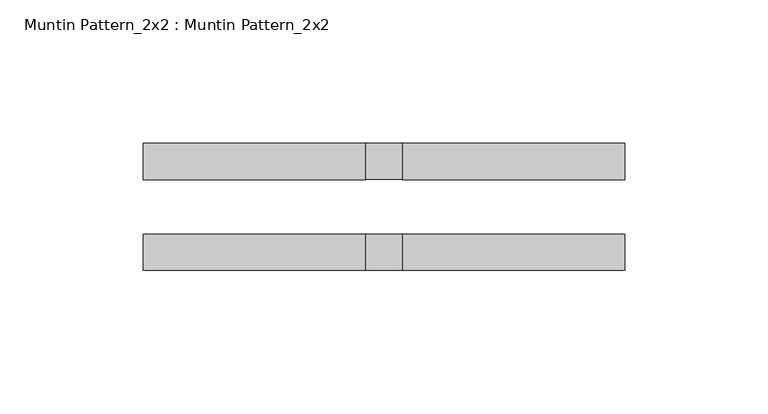
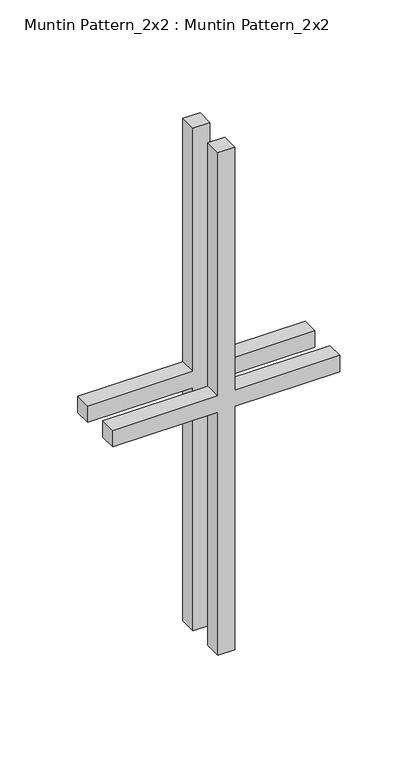
"""IFC4 building model written with IfcOpenShell, lengths in millimetres: proxy geometry, Muntin Pattern_2x2 : Muntin Pattern_2x2."""

from ifc_helpers import new_model, si_unit, frame, origin, place, context, project, spatial, polyline, outline, extrude, source, transform, mapped, element, save


def muntin_pattern_2x2_muntin_pattern_2x2_c179cf80(model_context):
    return source(origin(), model_context, "Body", "SweptSolid", [
        extrude(outline(polyline([(203.2, -6.35), (203.2, -84.1375), (190.5, -84.1375), (190.5, -6.35), (0.0, -6.35), (0.0, 6.35), (190.5, 6.35), (190.5, 84.1375), (203.2, 84.1375), (203.2, 6.35), (393.7, 6.35), (393.7, -6.35), (203.2, -6.35)])), frame((0.0, -22.225, 0.0), z_axis=(0.0, 1.0, 0.0), x_axis=(0.0, 0.0, 1.0)), (0.0, 0.0, 1.0), 12.7),
        extrude(outline(polyline([(203.2, -6.35), (203.2, -84.1375), (190.5, -84.1375), (190.5, -6.35), (0.0, -6.35), (0.0, 6.35), (190.5, 6.35), (190.5, 84.1375), (203.2, 84.1375), (203.2, 6.35), (393.7, 6.35), (393.7, -6.35), (203.2, -6.35)])), frame((0.0, 9.525, 0.0), z_axis=(0.0, 1.0, 0.0), x_axis=(0.0, 0.0, 1.0)), (0.0, 0.0, 1.0), 12.7),
    ])


if __name__ == "__main__":
    model = new_model("IFC4")
    model_context = context("Model", 3, world=origin())
    ifc_project = project(units=[si_unit("LENGTHUNIT", "METRE", prefix="MILLI")], contexts=[model_context])
    site = spatial("IfcSite", under=ifc_project)
    building = spatial("IfcBuilding", under=site)
    placement = place(None, origin())
    muntin_pattern_2x2_muntin_pattern_2x2_shape = muntin_pattern_2x2_muntin_pattern_2x2_c179cf80(model_context)
    element("IfcBuildingElementProxy", 1, Name="Muntin Pattern_2x2 : Muntin Pattern_2x2", ObjectType="Muntin Pattern_2x2 : Muntin Pattern_2x2", at=placement, inside=building, context=model_context, shape_type="MappedRepresentation", body=[
        mapped(muntin_pattern_2x2_muntin_pattern_2x2_shape, transform((0.0, 0.0, 0.0), x_axis=(1.0, 0.0, 0.0), y_axis=(0.0, 1.0, 0.0), z_axis=(0.0, 0.0, 1.0))),
    ])
    save(model, "model.ifc")

# Revit data of these elements
# Type "Muntin Pattern_2x2 : Muntin Pattern_2x2"
#   Width [instance default] = 4' - 0"
#   Thickness = 0' - 0 1/2"
#   Height [instance default] = 4' - 0"
#   Distance = 0' - 0 3/4"
#   Interior Material [instance default] = none
#   Exterior Material [instance default] = none
#   Default Elevation = 0
# Element 1 (IfcBuildingElementProxy, "Muntin Pattern_2x2 : Muntin Pattern_2x2")
#   Width = 0' - 6 5/8"
#   Height = 1' - 3 1/2"
#   Interior Material = Wood - Stained
#   Exterior Material = Clad - White
#   Materials on its faces: "Clad - White", "Wood - Stained"
# Materials
#   "Clad - White": class "Wood", colour RGB 242 242 238, transparency 0, Cost = 0
#   "Wood - Stained": class "Wood", colour RGB 224 178 126, transparency 0, Cost = 0
